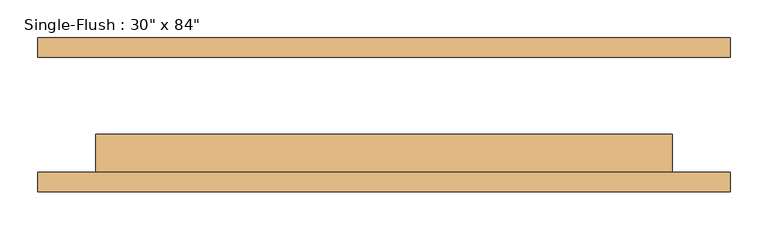
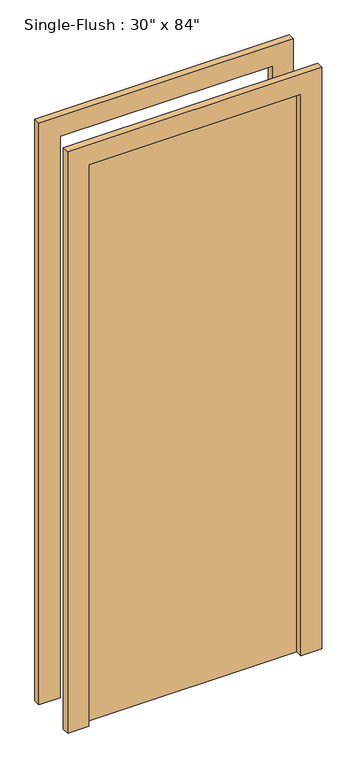
"""IFC4 building model written with IfcOpenShell, lengths in millimetres: door geometry."""

from ifc_helpers import new_model, si_unit, frame, origin, origin_with_axes, place, context, project, spatial, polyline, outline, extrude, source, transform, mapped, element, save


def door_e2b13fe9(model_context):
    return source(origin(), model_context, "Body", "SweptSolid", [
        extrude(outline(polyline([(2209.8, -457.2), (0.0, -457.2), (0.0, -381.0), (2133.6, -381.0), (2133.6, 381.0), (0.0, 381.0), (0.0, 457.2), (2209.8, 457.2), (2209.8, -457.2)])), frame((0.0, -101.6, 0.0), z_axis=(0.0, 1.0, 0.0), x_axis=(0.0, 0.0, 1.0)), (0.0, 0.0, 1.0), 25.4),
        extrude(outline(polyline([(2209.8, 457.2), (2209.8, -457.2), (0.0, -457.2), (0.0, -381.0), (2133.6, -381.0), (2133.6, 381.0), (0.0, 381.0), (0.0, 457.2), (2209.8, 457.2)])), frame((0.0, 76.2, 0.0), z_axis=(0.0, 1.0, 0.0), x_axis=(0.0, 0.0, 1.0)), (0.0, 0.0, 1.0), 25.4),
        extrude(outline(polyline([(381.0, -25.4), (381.0, -76.2), (-381.0, -76.2), (-381.0, -25.4), (381.0, -25.4)])), origin_with_axes(), (0.0, 0.0, 1.0), 2133.6),
    ])


if __name__ == "__main__":
    model = new_model("IFC4")
    model_context = context("Model", 3, world=origin())
    ifc_project = project(units=[si_unit("LENGTHUNIT", "METRE", prefix="MILLI")], contexts=[model_context])
    site = spatial("IfcSite", under=ifc_project)
    building = spatial("IfcBuilding", under=site)
    placement = place(None, origin())
    door_shape = door_e2b13fe9(model_context)
    element("IfcDoor", 1, ObjectType="Single-Flush : 30\" x 84\"", at=placement, inside=building, context=model_context, shape_type="MappedRepresentation", body=[
        mapped(door_shape, transform((0.0, 0.0, 0.0), x_axis=(1.0, 0.0, 0.0), y_axis=(0.0, 1.0, 0.0), z_axis=(0.0, 0.0, 1.0))),
    ])
    save(model, "model.ifc")

# Revit data of these elements
# Type "Single-Flush : 30\" x 84\""
#   Type Mark = "4"
#   Construction Type Id = "MDOOR"
#   Assembly Code = "C1020"
#   Analytic Construction = "Metal"
#   Thickness = 0' - 2"
#   Heat Transfer Coefficient (U) = 0.651978 BTU/(h·ft²·°F)
#   Height = 7' - 0"
#   Trim Projection Ext = 0' - 1"
#   Trim Projection Int = 0' - 1"
#   Trim Width = 0' - 3"
#   Width = 2' - 6"
#   Define Thermal Properties by = 1
#   Door Material = Door - Panel
#   Frame Material = Door - Frame
#   Visual Light Transmittance = 0
#   Solar Heat Gain Coefficient = 0
#   Function = (empty or 0)
#   Wall Closure = (empty or 0)
# Element 1 (IfcDoor, "Single-Flush : 30\" x 84\"")
#   Materials on its faces: "Door - Frame", "Door - Panel"
# Materials
#   "Door - Panel": class "Wood", colour RGB 210 159 95, transparency 0
#   "Door - Frame": colour RGB 118 70 51, transparency 0
